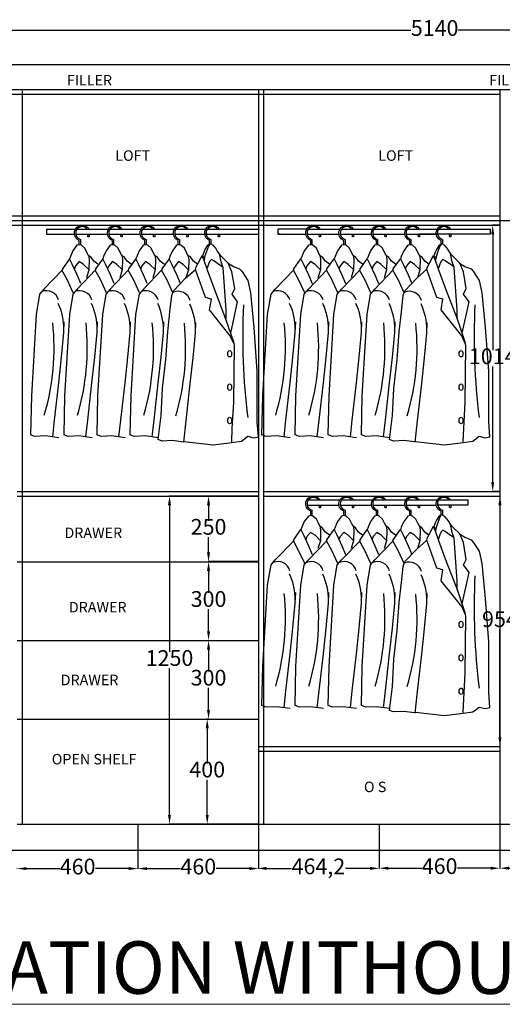
# Model space of a CAD drawing. Units: millimetres. Extents: x 1304 to 14372, y 283 to 7516.
# Tile 2 of 4: x 3237 to 5077, y 283 to 4036. Entities that reach past the tile are written whole.
import ezdxf

# ---------------------------------------------------------------- set-up
doc = ezdxf.new("R2010")
doc.units = ezdxf.units.MM
doc.layers.get('Defpoints').update_dxf_attribs({"color": 2})
for name, color, linetype, lineweight in [('A-ANNO-DIMS', 2, 'Continuous', 18), ('A-ANNO-TEXT', 3, 'Continuous', 18), ('A-FURN', 7, 'Continuous', 25)]:
    doc.layers.add(name, color=color, linetype=linetype, lineweight=lineweight)
doc.styles.get("Standard").update_dxf_attribs({"font": 'arial.ttf'})
doc.dimstyles.new('ISO-25', dxfattribs={"dimtxt": 60, "dimasz": 35, "dimexe": 1.25, "dimexo": 0.625, "dimtad": 0, "dimtih": 1, "dimtoh": 1, "dimtxsty": 'Standard', "dimcen": 2.5, "dimclrd": 1, "dimclre": 3, "dimadec": 0, "dimazin": 0, "dimtfac": 1, "dimtmove": 0, "dimatfit": 3, "dimfxl": 1, "dimarcsym": 0})

# ---------------------------------------------------------------- blocks, each defined once
blk = doc.blocks.new('*D16')
at = {"layer": 'A-ANNO-DIMS', "color": 0, "lineweight": -2, "transparency": 16777216}
for p, q in [((2248.6, 4008), (2248.6, 3995.4)), ((2283.6, 3996.6), (4728.5, 3996.6)), ((7353.6, 3996.6), (4908.8, 3996.6)), ((7388.6, 3865.9), (7388.6, 3997.9))]:
    blk.add_line(p, q, dxfattribs=at)
at = {"layer": 'A-ANNO-DIMS', "color": 0, "transparency": 16777216}
for points in [[(2283.6, 4002.4), (2283.6, 3990.8), (2248.6, 3996.6)], [(7353.6, 4002.4), (7353.6, 3990.8), (7388.6, 3996.6)]]:
    blk.add_solid(points, dxfattribs=at)
at = {"layer": 'Defpoints', "color": 0, "transparency": 16777216}
for p in [(2248.6, 4008.6), (7388.6, 3996.6), (7388.6, 3865.3)]:
    blk.add_point(p, dxfattribs=at)
at = {"layer": 'A-ANNO-DIMS', "color": 0, "transparency": 16777216, "insert": (4818.6, 3996.6), "char_height": 60, "attachment_point": 5}
blk.add_mtext('5140', dxfattribs=at)
blk = doc.blocks.new('*D18')
at = {"layer": 'A-ANNO-DIMS', "color": 0, "lineweight": -2, "transparency": 16777216}
for p, q in [((4147, 2220.3), (3955.4, 2220.3)), ((3956.7, 2185.3), (3956.7, 2126.5)), ((3956.7, 2005.3), (3956.7, 2064)), ((4147, 1970.3), (3955.4, 1970.3))]:
    blk.add_line(p, q, dxfattribs=at)
at = {"layer": 'A-ANNO-DIMS', "color": 0, "transparency": 16777216}
for points in [[(3950.8, 2185.3), (3962.5, 2185.3), (3956.7, 2220.3)], [(3950.8, 2005.3), (3962.5, 2005.3), (3956.7, 1970.3)]]:
    blk.add_solid(points, dxfattribs=at)
at = {"layer": 'Defpoints', "color": 0, "transparency": 16777216}
for p in [(4147.6, 2220.3), (3956.7, 1970.3), (4147.6, 1970.3)]:
    blk.add_point(p, dxfattribs=at)
at = {"layer": 'A-ANNO-DIMS', "color": 0, "transparency": 16777216, "insert": (3956.7, 2095.3), "char_height": 60, "attachment_point": 5}
blk.add_mtext('250', dxfattribs=at)
blk = doc.blocks.new('*D19')
at = {"layer": 'A-ANNO-DIMS', "color": 0, "lineweight": -2, "transparency": 16777216}
for p, q in [((3957.3, 1970.3), (3957.9, 1970.3)), ((3956.7, 1935.3), (3956.7, 1851.6)), ((3956.7, 1705.3), (3956.7, 1789)), ((3957.3, 1670.3), (3957.9, 1670.3))]:
    blk.add_line(p, q, dxfattribs=at)
at = {"layer": 'A-ANNO-DIMS', "color": 0, "transparency": 16777216}
for points in [[(3950.8, 1935.3), (3962.5, 1935.3), (3956.7, 1970.3)], [(3950.8, 1705.3), (3962.5, 1705.3), (3956.7, 1670.3)]]:
    blk.add_solid(points, dxfattribs=at)
at = {"layer": 'Defpoints', "color": 0, "transparency": 16777216}
for p in [(3956.7, 1970.3), (3956.7, 1670.3), (3956.7, 1670.3)]:
    blk.add_point(p, dxfattribs=at)
at = {"layer": 'A-ANNO-DIMS', "color": 0, "transparency": 16777216, "insert": (3956.7, 1820.3), "char_height": 60, "attachment_point": 5}
blk.add_mtext('300', dxfattribs=at)
blk = doc.blocks.new('*D20')
at = {"layer": 'A-ANNO-DIMS', "color": 0, "lineweight": -2, "transparency": 16777216}
for p, q in [((3957.3, 1670.3), (3957.9, 1670.3)), ((3956.7, 1635.3), (3956.7, 1551.6)), ((3956.7, 1405.3), (3956.7, 1489)), ((3957.3, 1370.3), (3957.9, 1370.3))]:
    blk.add_line(p, q, dxfattribs=at)
at = {"layer": 'A-ANNO-DIMS', "color": 0, "transparency": 16777216}
for points in [[(3950.8, 1635.3), (3962.5, 1635.3), (3956.7, 1670.3)], [(3950.8, 1405.3), (3962.5, 1405.3), (3956.7, 1370.3)]]:
    blk.add_solid(points, dxfattribs=at)
at = {"layer": 'Defpoints', "color": 0, "transparency": 16777216}
for p in [(3956.7, 1670.3), (3956.7, 1370.3), (3956.7, 1370.3)]:
    blk.add_point(p, dxfattribs=at)
at = {"layer": 'A-ANNO-DIMS', "color": 0, "transparency": 16777216, "insert": (3956.7, 1520.3), "char_height": 60, "attachment_point": 5}
blk.add_mtext('300', dxfattribs=at)
blk = doc.blocks.new('*D21')
at = {"layer": 'A-ANNO-DIMS', "color": 0, "lineweight": -2, "transparency": 16777216}
for p, q in [((3957.3, 1370.3), (3950.3, 1370.3)), ((3951.6, 1335.3), (3951.6, 1201.5)), ((3951.6, 1005.3), (3951.6, 1139)), ((3957.3, 970.3), (3950.3, 970.3))]:
    blk.add_line(p, q, dxfattribs=at)
at = {"layer": 'A-ANNO-DIMS', "color": 0, "transparency": 16777216}
for points in [[(3945.7, 1335.3), (3957.4, 1335.3), (3951.6, 1370.3)], [(3945.7, 1005.3), (3957.4, 1005.3), (3951.6, 970.3)]]:
    blk.add_solid(points, dxfattribs=at)
at = {"layer": 'Defpoints', "color": 0, "transparency": 16777216}
for p in [(3957.9, 1370.3), (3951.6, 970.3), (3957.9, 970.3)]:
    blk.add_point(p, dxfattribs=at)
at = {"layer": 'A-ANNO-DIMS', "color": 0, "transparency": 16777216, "insert": (3951.6, 1170.3), "char_height": 60, "attachment_point": 5}
blk.add_mtext('400', dxfattribs=at)
blk = doc.blocks.new('*D22')
at = {"layer": 'A-ANNO-DIMS', "color": 0, "lineweight": -2, "transparency": 16777216}
for p, q in [((4147, 2220.3), (3806.5, 2220.3)), ((3807.8, 2185.3), (3807.8, 1626.5)), ((3807.8, 1005.3), (3807.8, 1564)), ((4147, 970.3), (3806.5, 970.3))]:
    blk.add_line(p, q, dxfattribs=at)
at = {"layer": 'A-ANNO-DIMS', "color": 0, "transparency": 16777216}
for points in [[(3801.9, 2185.3), (3813.6, 2185.3), (3807.8, 2220.3)], [(3801.9, 1005.3), (3813.6, 1005.3), (3807.8, 970.3)]]:
    blk.add_solid(points, dxfattribs=at)
at = {"layer": 'Defpoints', "color": 0, "transparency": 16777216}
for p in [(4147.6, 2220.3), (3807.8, 970.3), (4147.6, 970.3)]:
    blk.add_point(p, dxfattribs=at)
at = {"layer": 'A-ANNO-DIMS', "color": 0, "transparency": 16777216, "insert": (3807.8, 1595.3), "char_height": 60, "attachment_point": 5}
blk.add_mtext('1250', dxfattribs=at)
blk = doc.blocks.new('*D23')
at = {"layer": 'A-ANNO-DIMS', "color": 0, "lineweight": -2, "transparency": 16777216}
for p, q in [((5067, 3252.3), (5038.8, 3252.3)), ((5040.1, 3217.3), (5040.1, 2776.5)), ((5040.1, 2273.3), (5040.1, 2714)), ((5067, 2238.3), (5038.8, 2238.3))]:
    blk.add_line(p, q, dxfattribs=at)
at = {"layer": 'A-ANNO-DIMS', "color": 0, "transparency": 16777216}
for points in [[(5034.2, 3217.3), (5045.9, 3217.3), (5040.1, 3252.3)], [(5034.2, 2273.3), (5045.9, 2273.3), (5040.1, 2238.3)]]:
    blk.add_solid(points, dxfattribs=at)
at = {"layer": 'Defpoints', "color": 0, "transparency": 16777216}
for p in [(5067.6, 3252.3), (5040.1, 2238.3), (5067.6, 2238.3)]:
    blk.add_point(p, dxfattribs=at)
at = {"layer": 'A-ANNO-DIMS', "color": 0, "transparency": 16777216, "insert": (5040.1, 2745.3), "char_height": 60, "attachment_point": 5}
blk.add_mtext('1014', dxfattribs=at)
blk = doc.blocks.new('*D24')
at = {"layer": 'A-ANNO-DIMS', "color": 0, "lineweight": -2, "transparency": 16777216}
for p, q in [((5068.3, 2220.3), (5068.9, 2220.3)), ((5067.6, 2185.3), (5067.6, 1774.5)), ((5067.6, 1301.3), (5067.6, 1712)), ((5068.3, 1266.3), (5068.9, 1266.3))]:
    blk.add_line(p, q, dxfattribs=at)
at = {"layer": 'A-ANNO-DIMS', "color": 0, "transparency": 16777216}
for points in [[(5061.8, 2185.3), (5073.5, 2185.3), (5067.6, 2220.3)], [(5061.8, 1301.3), (5073.5, 1301.3), (5067.6, 1266.3)]]:
    blk.add_solid(points, dxfattribs=at)
at = {"layer": 'Defpoints', "color": 0, "transparency": 16777216}
for p in [(5067.6, 2220.3), (5067.6, 1266.3), (5067.6, 1266.3)]:
    blk.add_point(p, dxfattribs=at)
at = {"layer": 'A-ANNO-DIMS', "color": 0, "transparency": 16777216, "insert": (5067.6, 1743.3), "char_height": 60, "attachment_point": 5}
blk.add_mtext('954', dxfattribs=at)
blk = doc.blocks.new('*D36')
at = {"layer": 'A-ANNO-DIMS', "color": 0, "lineweight": -2, "transparency": 16777216}
for p, q in [((3227.6, 801.1), (3227.6, 801.7)), ((3262.6, 800.5), (3389.6, 800.5)), ((3652.6, 800.5), (3525.7, 800.5)), ((3687.6, 801.1), (3687.6, 801.7))]:
    blk.add_line(p, q, dxfattribs=at)
at = {"layer": 'A-ANNO-DIMS', "color": 0, "transparency": 16777216}
for points in [[(3262.6, 806.3), (3262.6, 794.7), (3227.6, 800.5)], [(3652.6, 806.3), (3652.6, 794.7), (3687.6, 800.5)]]:
    blk.add_solid(points, dxfattribs=at)
at = {"layer": 'Defpoints', "color": 0, "transparency": 16777216}
for p in [(3227.6, 800.5), (3687.6, 800.5), (3687.6, 800.5)]:
    blk.add_point(p, dxfattribs=at)
at = {"layer": 'A-ANNO-DIMS', "color": 0, "transparency": 16777216, "insert": (3457.6, 800.5), "char_height": 60, "attachment_point": 5}
blk.add_mtext('460', dxfattribs=at)
blk = doc.blocks.new('*D37')
at = {"layer": 'A-ANNO-DIMS', "color": 0, "lineweight": -2, "transparency": 16777216}
for p, q in [((4143.4, 801.8), (4143.4, 802.4)), ((4178.4, 801.2), (4272.8, 801.2)), ((4572.6, 801.2), (4478.3, 801.2)), ((4607.6, 801.8), (4607.6, 802.4))]:
    blk.add_line(p, q, dxfattribs=at)
at = {"layer": 'A-ANNO-DIMS', "color": 0, "transparency": 16777216}
for points in [[(4178.4, 807), (4178.4, 795.4), (4143.4, 801.2)], [(4572.6, 807), (4572.6, 795.4), (4607.6, 801.2)]]:
    blk.add_solid(points, dxfattribs=at)
at = {"layer": 'Defpoints', "color": 0, "transparency": 16777216}
for p in [(4143.4, 801.2), (4607.6, 801.2), (4607.6, 801.2)]:
    blk.add_point(p, dxfattribs=at)
at = {"layer": 'A-ANNO-DIMS', "color": 0, "transparency": 16777216, "insert": (4375.5, 801.2), "char_height": 60, "attachment_point": 5}
blk.add_mtext('464,2', dxfattribs=at)
blk = doc.blocks.new('*D38')
at = {"layer": 'A-ANNO-DIMS', "color": 0, "lineweight": -2, "transparency": 16777216}
for p, q in [((4607.6, 969.7), (4607.6, 800.7)), ((5067.6, 969.7), (5067.6, 800.7)), ((4642.6, 802), (4769.6, 802)), ((5032.6, 802), (4905.7, 802))]:
    blk.add_line(p, q, dxfattribs=at)
at = {"layer": 'A-ANNO-DIMS', "color": 0, "transparency": 16777216}
for points in [[(4642.6, 807.8), (4642.6, 796.1), (4607.6, 802)], [(5032.6, 807.8), (5032.6, 796.1), (5067.6, 802)]]:
    blk.add_solid(points, dxfattribs=at)
at = {"layer": 'Defpoints', "color": 0, "transparency": 16777216}
for p in [(4607.6, 970.3), (5067.6, 970.3), (5067.6, 802)]:
    blk.add_point(p, dxfattribs=at)
at = {"layer": 'A-ANNO-DIMS', "color": 0, "transparency": 16777216, "insert": (4837.6, 802), "char_height": 60, "attachment_point": 5}
blk.add_mtext('460', dxfattribs=at)
blk = doc.blocks.new('*D39')
at = {"layer": 'A-ANNO-DIMS', "color": 0, "lineweight": -2, "transparency": 16777216}
for p, q in [((5067.6, 969.7), (5067.6, 800.7)), ((5527.6, 969.7), (5527.6, 800.7)), ((5102.6, 802), (5229.6, 802)), ((5492.6, 802), (5365.7, 802))]:
    blk.add_line(p, q, dxfattribs=at)
at = {"layer": 'A-ANNO-DIMS', "color": 0, "transparency": 16777216}
for points in [[(5102.6, 807.8), (5102.6, 796.1), (5067.6, 802)], [(5492.6, 807.8), (5492.6, 796.1), (5527.6, 802)]]:
    blk.add_solid(points, dxfattribs=at)
at = {"layer": 'Defpoints', "color": 0, "transparency": 16777216}
for p in [(5067.6, 970.3), (5527.6, 970.3), (5527.6, 802)]:
    blk.add_point(p, dxfattribs=at)
at = {"layer": 'A-ANNO-DIMS', "color": 0, "transparency": 16777216, "insert": (5297.6, 802), "char_height": 60, "attachment_point": 5}
blk.add_mtext('460', dxfattribs=at)
blk = doc.blocks.new('*D44')
at = {"layer": 'A-ANNO-DIMS', "color": 0, "lineweight": -2, "transparency": 16777216}
for p, q in [((3687.6, 969.7), (3687.6, 799.2)), ((4147.6, 969.7), (4147.6, 799.2)), ((3722.6, 800.5), (3849.6, 800.5)), ((4112.6, 800.5), (3985.7, 800.5))]:
    blk.add_line(p, q, dxfattribs=at)
at = {"layer": 'A-ANNO-DIMS', "color": 0, "transparency": 16777216}
for points in [[(3722.6, 806.3), (3722.6, 794.7), (3687.6, 800.5)], [(4112.6, 806.3), (4112.6, 794.7), (4147.6, 800.5)]]:
    blk.add_solid(points, dxfattribs=at)
at = {"layer": 'Defpoints', "color": 0, "transparency": 16777216}
for p in [(3687.6, 970.3), (4147.6, 970.3), (3687.6, 800.5)]:
    blk.add_point(p, dxfattribs=at)
at = {"layer": 'A-ANNO-DIMS', "color": 0, "transparency": 16777216, "insert": (3917.6, 800.5), "char_height": 60, "attachment_point": 5}
blk.add_mtext('460', dxfattribs=at)
blk = doc.blocks.new('CLOTHES-HANGING')
for p, q in [((4337.7, 3238.2), (4457.6, 3238.2)), ((4463.8, 3238.2), (4582, 3238.2)), ((4588.1, 3238.2), (4709.1, 3238.2)), ((4715.2, 3238.2), (4828.6, 3238.2)), ((4332.7, 3218.2), (4453.7, 3218.2)), ((4458.7, 3218.2), (4578, 3218.2)), ((4583.1, 3218.2), (4705.1, 3218.2)), ((4710.2, 3218.2), (4824.6, 3218.2))]:
    blk.add_line(p, q)
for points in [[(4346, 3177.2), (4346, 3194.9, -0.375799), (4328.2, 3230.2, -0.662316), (4381.8, 3238.2), (4421.2, 3238.2)], [(4375.7, 3238.2, 0.616313), (4333.1, 3229, 0.413702), (4351, 3198.5), (4351, 3177.2)], [(4472, 3177.2), (4472, 3194.9, -0.375799), (4454.3, 3230.2, -0.662316), (4507.9, 3238.2)], [(4501.8, 3238.2, 0.616313), (4459.1, 3229, 0.413702), (4477, 3198.5), (4477, 3177.2)], [(4596.4, 3177.2), (4596.4, 3194.9, -0.375799), (4578.7, 3230.2, -0.662316), (4632.3, 3238.2)], [(4626.1, 3238.2, 0.616313), (4583.5, 3229, 0.413702), (4601.4, 3198.5), (4601.4, 3177.2)], [(4723.5, 3177.6), (4723.5, 3194.9, -0.375799), (4705.7, 3230.2, -0.662316), (4759.3, 3238.2)], [(4753.2, 3238.2, 0.616313), (4710.6, 3229, 0.413702), (4728.5, 3198.5), (4728.5, 3178)], [(4843, 3179.9), (4843, 3194.9, -0.375799), (4825.2, 3230.2, -0.662316), (4878.8, 3238.2)], [(4872.7, 3238.2, 0.616313), (4830.1, 3229, 0.413702), (4848, 3198.5), (4848, 3180.3)], [(4383.5, 3218.2, -0.068798), (4383.9, 3210.2, -1.055238), (4378.9, 3210.6, 0.07858), (4378.4, 3218.2, 0.07858)], [(4509.5, 3218.2, -0.068798), (4509.9, 3210.2, -1.055238), (4504.9, 3210.6, 0.07858), (4504.4, 3218.2)], [(4633.9, 3218.2, -0.068798), (4634.3, 3210.2, -1.055238), (4629.3, 3210.6, 0.07858), (4628.8, 3218.2)], [(4761, 3218.2, -0.068798), (4761.4, 3210.2, -1.055238), (4756.4, 3210.6, 0.07858), (4755.9, 3218.2)], [(4880.4, 3218.2, -0.068798), (4880.8, 3210.2, -1.055238), (4875.8, 3210.6, 0.07858), (4875.3, 3218.2)]]:
    blk.add_lwpolyline(points, format="xyb")
for points in [[(4381.1, 3137), (4375.4, 3148.9), (4367.7, 3164.8), (4354.3, 3176.3), (4346.7, 3178.2), (4337.1, 3176.3), (4321.8, 3155.3), (4312.3, 3133.6), (4309.1, 3124)], [(4507.8, 3137), (4502, 3148.9), (4494.4, 3164.8), (4481, 3176.3), (4473.3, 3178.2), (4463.8, 3176.3), (4448.5, 3155.3), (4438.9, 3133.6), (4435.7, 3124)], [(4633.8, 3137), (4628.1, 3148.9), (4620.4, 3164.8), (4607, 3176.3), (4599.4, 3178.2), (4589.8, 3176.3), (4574.5, 3155.3), (4565, 3133.6), (4561.8, 3124)], [(4760.5, 3137), (4754.7, 3148.9), (4747.1, 3164.8), (4733.7, 3176.3), (4726, 3178.2), (4716.5, 3176.3), (4701.2, 3155.3), (4691.6, 3133.6), (4688.4, 3124)], [(4844.1, 3180.6), (4834, 3174), (4825.2, 3160.3), (4820.3, 3149.8), (4815.3, 3134.5)], [(4905.1, 2895.5), (4905.1, 2928.3), (4893.2, 3092), (4885.8, 3113.6), (4879.5, 3145.3), (4872.3, 3155.4), (4866.4, 3164.6), (4857.9, 3174.7), (4848.7, 3179.9), (4844.1, 3180.6), (4838.9, 3172.4), (4830.7, 3152.1), (4825.2, 3135.8), (4821.9, 3121.7), (4821.6, 3119.8)], [(4268.3, 2442.4), (4216.9, 2449.4), (4176.8, 2447.6), (4160, 2453.9), (4163.3, 2602.1), (4181.5, 2912.1), (4194.8, 2990.1), (4211.2, 3009.3), (4281.6, 3082.3), (4281.6, 3085.9), (4309, 3124.3), (4319, 3104.2), (4338.2, 3063.1), (4352.3, 3030.2)], [(4395, 2442.4), (4343.5, 2449.4), (4303.4, 2447.6), (4286.6, 2453.9), (4289.9, 2602.1), (4308.2, 2912.1), (4321.5, 2990.1), (4337.9, 3009.3), (4408.2, 3082.3), (4408.2, 3085.9), (4435.6, 3124.3), (4445.7, 3104.2), (4464.8, 3063.1), (4479, 3030.2)], [(4417.3, 3103.8), (4402.1, 3115.1), (4390.2, 3131.6), (4381.1, 3137), (4383.9, 3123.3), (4382.9, 3082.3), (4373.4, 3051.9)], [(4521, 2442.4), (4469.6, 2449.4), (4429.5, 2447.6), (4412.7, 2453.9), (4416, 2602.1), (4434.2, 2912.1), (4447.5, 2990.1), (4463.9, 3009.3), (4534.3, 3082.3), (4534.3, 3085.9), (4561.7, 3124.3), (4571.7, 3104.2), (4590.9, 3063.1), (4605, 3030.2)], [(4543.9, 3103.8), (4528.8, 3115.1), (4516.9, 3131.6), (4507.8, 3137), (4510.5, 3123.3), (4509.6, 3082.3), (4500.1, 3051.9)], [(4647.7, 2442.4), (4596.2, 2449.4), (4556.1, 2447.6), (4539.3, 2453.9), (4542.6, 2602.1), (4560.9, 2912.1), (4574.2, 2990.1), (4590.6, 3009.3), (4660.9, 3082.3), (4660.9, 3085.9), (4688.3, 3124.3), (4698.4, 3104.2), (4717.5, 3063.1), (4731.7, 3030.2)], [(4670, 3103.8), (4654.8, 3115.1), (4642.9, 3131.6), (4633.8, 3137), (4636.6, 3123.3), (4635.6, 3082.3), (4626.1, 3051.9)], [(4741.7, 2426.4), (4701.6, 2431.8), (4661.5, 2430), (4646.8, 2435.5), (4657.7, 2527.1), (4662.8, 2630.8), (4676.4, 2741.2), (4683.2, 2846.6), (4691.7, 2923.1), (4698.5, 2984.2), (4705.3, 3002.9), (4751.3, 3050.5), (4788.7, 3084.5), (4791.6, 3094), (4800.3, 3110.8), (4810.1, 3129.9), (4814.2, 3136.2), (4822.9, 3129.9), (4824, 3129.3)], [(4796.6, 3103.8), (4781.5, 3115.1), (4769.6, 3131.6), (4760.5, 3137), (4763.2, 3123.3), (4762.3, 3082.3), (4752.8, 3051.9)], [(4813, 3134.5), (4820.5, 3120), (4833.9, 3083), (4858.8, 3013.5), (4903.9, 2896.1), (4934, 2808.5), (4936.1, 2793.8), (4933.4, 2577.1), (4928.1, 2479.6), (4926.4, 2426.9)], [(4891.3, 3093.9), (4878.5, 3102.4), (4858.9, 3116.8), (4850.4, 3122.1), (4843.8, 3115.8), (4838.3, 3104.7), (4834.7, 3092.6), (4833.3, 3088.4)], [(4923.7, 2841.2), (4949.8, 2961), (4929, 2990.1), (4939.4, 3010.9), (4928.2, 3074.9), (4914.1, 3108.4), (4888.7, 3132.9), (4877.6, 3145.6)], [(4323.2, 2995.2), (4300.2, 3045.3), (4280.1, 3081.8)], [(4383.7, 3082), (4362.6, 3103), (4345.4, 3113.9), (4332, 3097.9), (4327.4, 3086.3)], [(4449.8, 2995.2), (4426.8, 3045.3), (4406.8, 3081.8)], [(4510.3, 3082), (4489.3, 3103), (4472.1, 3113.9), (4458.7, 3097.9), (4454, 3086.3)], [(4575.9, 2995.2), (4552.9, 3045.3), (4532.8, 3081.8)], [(4636.4, 3082), (4615.3, 3103), (4598.1, 3113.9), (4584.7, 3097.9), (4580.1, 3086.3)], [(4702.5, 2995.2), (4679.5, 3045.3), (4659.4, 3081.8)], [(4763, 3082), (4742, 3103), (4724.8, 3113.9), (4711.4, 3097.9), (4706.7, 3086.3)], [(4935, 2802.3), (4921.9, 2831), (4842.9, 2929.7), (4849.5, 2970.8), (4827.3, 2977.3), (4789.4, 3084.2)], [(4913.3, 3108.4), (4934.2, 3095.7), (4957.3, 3086), (4965.4, 3077.1), (4988.3, 3042.5), (4998.2, 2994.9), (5011, 2862.2), (5023.4, 2696.6), (5023.4, 2503.8), (5027.9, 2446.2)], [(4244.7, 2445.6), (4251.6, 2509.4), (4267.7, 2651.6), (4278.3, 2749.4), (4287.2, 2843.6), (4289, 2884.5)], [(4371.4, 2445.6), (4378.3, 2509.4), (4394.3, 2651.6), (4405, 2749.4), (4413.9, 2843.6), (4415.7, 2884.5)], [(4497.4, 2445.6), (4504.3, 2509.4), (4520.4, 2651.6), (4531, 2749.4), (4539.9, 2843.6), (4541.7, 2884.5)], [(4624, 2445.6), (4631, 2509.4), (4647, 2651.6), (4657.7, 2749.4), (4666.6, 2843.6), (4668.4, 2884.5)], [(4744.4, 2425.4), (4753.3, 2507.2), (4769.3, 2649.4), (4779.9, 2747.1), (4788.8, 2841.3), (4790.6, 2882.2)], [(4745.3, 2428.2), (4856.5, 2415.4), (4927.6, 2424.5), (4964.1, 2430), (4988.3, 2448.2), (5011.3, 2442.8), (5029, 2446.4)]]:
    blk.add_lwpolyline(points)
for centre, radius, start, end in [((4220.5, 2954.5), 48.4, 15.7523, 111.1565), ((4347.2, 2954.5), 48.4, 15.7523, 111.1565), ((4473.2, 2954.5), 48.4, 15.7523, 111.1565), ((4599.9, 2954.5), 48.4, 15.7523, 111.1565), ((4722.1, 2952.3), 48.4, 15.7523, 111.1565), ((4054.1, 2856), 233.4, 359.9116, 24.988), ((4180.8, 2856), 233.4, 359.9116, 24.988), ((4306.8, 2856), 233.4, 359.9116, 24.988), ((4433.5, 2856), 233.4, 359.9116, 24.988), ((4555.7, 2853.8), 233.4, 359.9116, 24.988), ((7480.3, 2829.3), 2511.1, 177.2767, 187.0811), ((3340.3, 2786.1), 909.7, 343.5409, 5.9886), ((3466.9, 2786.1), 909.7, 343.5409, 5.9886), ((3719.6, 2786.1), 909.7, 343.5409, 5.9886), ((3841.9, 2783.9), 909.7, 343.5409, 5.9886)]:
    blk.add_arc(centre, radius, start, end)
for centre in [(4919.4, 2762.9), (4919.4, 2635.5), (4919.4, 2508.1)]:
    blk.add_ellipse(centre, major_axis=(0, 12.4), ratio=0.580645)

msp = doc.modelspace()

# ---------------------------------------------------------------- linework, layer by layer
at = {"layer": 'A-FURN'}
for p, q in [((2018.643, 3865.285), (7618.643, 3865.285)), ((2316.643, 3770.285), (7388.643, 3770.285)), ((3245.643, 3765.285), (3245.643, 970.285)), ((4147.643, 3770.285), (4147.643, 970.285)), ((4165.643, 3770.285), (4165.643, 970.285)), ((5067.643, 3770.285), (5067.643, 970.285)), ((2316.643, 3752.285), (5067.643, 3752.285)), ((2316.643, 3288.285), (5067.643, 3288.285)), ((2316.643, 3270.285), (5545.643, 3270.285)), ((2316.643, 3252.285), (4165.643, 3252.285)), ((3339.108, 3238.199), (3449.429, 3238.199)), ((3339.108, 3238.199), (3339.108, 3218.199)), ((3455.532, 3238.199), (3575.461, 3238.199)), ((3499.644, 3238.199), (3538.99, 3238.199)), ((3581.563, 3238.199), (3699.848, 3238.199)), ((3705.951, 3238.199), (3826.926, 3238.199)), ((3833.029, 3238.199), (3946.395, 3238.199)), ((3881.136, 3238.199), (4147.643, 3238.199)), ((4165.643, 3252.285), (5067.643, 3252.285)), ((3339.108, 3218.199), (3445.437, 3218.199)), ((3450.506, 3218.199), (3571.468, 3218.199)), ((3576.537, 3218.199), (3695.856, 3218.199)), ((3700.925, 3218.199), (3822.934, 3218.199)), ((3828.003, 3218.199), (3942.403, 3218.199)), ((3876.11, 3218.199), (4147.643, 3218.199)), ((4229.579, 3218.199), (4221.295, 3218.199)), ((3227.643, 2238.285), (4147.643, 2238.285)), ((3227.643, 2220.285), (4147.643, 2220.285)), ((4165.643, 2238.285), (5067.643, 2238.285)), ((4165.643, 2220.285), (5067.643, 2220.285)), ((4945.153, 2186.199), (4829.663, 2186.177)), ((4834.685, 2206.199), (4945.153, 2206.199)), ((4945.153, 2206.199), (4945.153, 2186.199)), ((3227.643, 1970.285), (4147.643, 1970.285)), ((3227.643, 1670.285), (4147.643, 1670.285)), ((3227.643, 1370.285), (4147.643, 1370.285)), ((4147.643, 1266.285), (5067.643, 1266.285)), ((4147.643, 1248.285), (5067.643, 1248.285)), ((3227.643, 970.285), (4147.643, 970.285)), ((4147.643, 970.285), (5527.643, 970.285)), ((2018.643, 870.285), (7618.643, 870.285))]:
    msp.add_line(p, q, dxfattribs=at)
for points in [[(3463.826, 3177.2), (3463.826, 3194.87, -0.37579854), (3446.056, 3230.24, -0.66231577), (3499.644, 3238.199, -0.66231577)], [(3493.542, 3238.199, 0.61631348), (3450.897, 3228.987, 0.41370242), (3468.826, 3198.466), (3468.826, 3177.234)], [(3589.858, 3177.2), (3589.858, 3194.87, -0.37579854), (3572.088, 3230.24, -0.66231577), (3625.676, 3238.199)], [(3619.573, 3238.199, 0.61631348), (3576.928, 3228.987, 0.41370242), (3594.858, 3198.466), (3594.858, 3177.234)], [(3714.245, 3177.2), (3714.245, 3194.87, -0.37579854), (3696.475, 3230.24, -0.66231577), (3750.063, 3238.199)], [(3743.961, 3238.199, 0.61631348), (3701.316, 3228.987, 0.41370242), (3719.245, 3198.466), (3719.245, 3177.234)], [(3841.323, 3177.573), (3841.323, 3194.87, -0.37579854), (3823.554, 3230.24, -0.66231577), (3877.141, 3238.199)], [(3871.039, 3238.199, 0.61631348), (3828.394, 3228.987, 0.41370242), (3846.323, 3198.466), (3846.323, 3177.951)], [(3960.792, 3179.875), (3960.792, 3194.87, -0.37579854), (3943.022, 3230.24, -0.66231577), (3996.61, 3238.199)], [(3990.508, 3238.199, 0.61631348), (3947.863, 3228.987, 0.41370242), (3965.792, 3198.466), (3965.792, 3180.349)], [(3501.277, 3218.199, -0.06879847), (3501.677, 3210.151, -1.05523784), (3496.696, 3210.589, 0.07858039), (3496.169, 3218.199, 0.07858039)], [(3627.308, 3218.199, -0.06879847), (3627.709, 3210.151, -1.05523784), (3622.728, 3210.589, 0.07858039), (3622.201, 3218.199)], [(3751.696, 3218.199, -0.06879847), (3752.096, 3210.151, -1.05523784), (3747.115, 3210.589, 0.07858039), (3746.588, 3218.199)], [(3878.774, 3218.199, -0.06879847), (3879.174, 3210.151, -1.05523784), (3874.193, 3210.589, 0.07858039), (3873.666, 3218.199)], [(3998.242, 3218.199, -0.06879847), (3998.643, 3210.151, -1.05523784), (3993.662, 3210.589, 0.07858039), (3993.135, 3218.199)]]:
    msp.add_lwpolyline(points, format="xyb", dxfattribs=at)
for points in [[(4331.617, 3238.199), (4221.295, 3238.199), (4221.295, 3218.199), (4327.624, 3218.199)], [(4763.323, 3238.199), (5029.83, 3238.199), (5029.83, 3218.199), (4758.297, 3218.199)], [(3498.925, 3137.031), (3493.189, 3148.886), (3485.539, 3164.81), (3472.151, 3176.276), (3464.501, 3178.186), (3454.939, 3176.276), (3439.639, 3155.256), (3430.076, 3133.599), (3426.889, 3124.045)], [(3625.574, 3137.031), (3619.837, 3148.886), (3612.187, 3164.81), (3598.8, 3176.276), (3591.15, 3178.186), (3581.587, 3176.276), (3566.287, 3155.256), (3556.725, 3133.599), (3553.537, 3124.045)], [(3751.624, 3137.031), (3745.887, 3148.886), (3738.237, 3164.81), (3724.85, 3176.276), (3717.2, 3178.186), (3707.637, 3176.276), (3692.337, 3155.256), (3682.775, 3133.599), (3679.587, 3124.045)], [(3878.272, 3137.031), (3872.536, 3148.886), (3864.886, 3164.81), (3851.498, 3176.276), (3843.848, 3178.186), (3834.286, 3176.276), (3818.986, 3155.256), (3809.423, 3133.599), (3806.236, 3124.045)], [(3961.959, 3180.587), (3951.813, 3174.046), (3942.976, 3160.312), (3938.066, 3149.847), (3933.157, 3134.477)], [(3997.307, 3145.269), (3990.107, 3155.406), (3984.215, 3164.563), (3975.705, 3174.7), (3966.541, 3179.933), (3961.959, 3180.587), (3956.722, 3172.411), (3948.54, 3152.136), (3942.976, 3135.785), (3939.703, 3121.723), (3939.375, 3119.761)], [(3470.126, 3030.195), (3456.003, 3063.121), (3436.825, 3104.182), (3426.779, 3124.256), (3399.381, 3085.933), (3399.381, 3082.283), (3329.062, 3009.285), (3312.623, 2990.123), (3299.345, 2912.137), (3281.091, 2602.085), (3277.795, 2453.884)], [(3596.774, 3030.195), (3582.651, 3063.121), (3563.473, 3104.182), (3553.427, 3124.256), (3526.03, 3085.933), (3526.03, 3082.283), (3455.71, 3009.285), (3439.272, 2990.123), (3425.993, 2912.137), (3407.739, 2602.085), (3404.443, 2453.884)], [(3535.105, 3103.76), (3519.93, 3115.132), (3508.058, 3131.556), (3498.925, 3137.031), (3501.665, 3123.344), (3500.752, 3082.283), (3491.243, 3051.881)], [(3722.824, 3030.195), (3708.701, 3063.121), (3689.523, 3104.182), (3679.477, 3124.256), (3652.08, 3085.933), (3652.08, 3082.283), (3581.76, 3009.285), (3565.322, 2990.123), (3552.043, 2912.137), (3533.789, 2602.085), (3530.493, 2453.884)], [(3661.753, 3103.76), (3646.578, 3115.132), (3634.706, 3131.556), (3625.574, 3137.031), (3628.313, 3123.344), (3627.4, 3082.283), (3617.892, 3051.881)], [(3849.473, 3030.195), (3835.35, 3063.121), (3816.171, 3104.182), (3806.126, 3124.256), (3778.728, 3085.933), (3778.728, 3082.283), (3708.409, 3009.285), (3691.97, 2990.123), (3678.692, 2912.137), (3660.438, 2602.085), (3657.142, 2453.884)], [(3787.803, 3103.76), (3772.628, 3115.132), (3760.756, 3131.556), (3751.624, 3137.031), (3754.363, 3123.344), (3753.45, 3082.283), (3743.942, 3051.881)], [(3764.654, 2435.499), (3775.536, 2527.141), (3780.638, 2630.794), (3794.244, 2741.244), (3801.046, 2846.596), (3809.55, 2923.061), (3816.352, 2984.234), (3823.155, 3002.925), (3869.073, 3050.504), (3906.488, 3084.488), (3909.388, 3093.978), (3918.076, 3110.76), (3927.922, 3129.857), (3931.976, 3136.223), (3940.664, 3129.857), (3941.822, 3129.278)], [(3914.452, 3103.76), (3899.277, 3115.132), (3887.404, 3131.556), (3878.272, 3137.031), (3881.012, 3123.344), (3880.099, 3082.283), (3870.59, 3051.881)], [(3930.818, 3134.486), (3938.347, 3120.019), (3951.668, 3082.983), (3976.574, 3013.539), (4021.75, 2896.064), (4051.839, 2808.498), (4053.908, 2793.752), (4051.175, 2577.069), (4045.943, 2479.562), (4044.243, 2426.886)], [(4009.09, 3093.926), (3996.325, 3102.429), (3976.687, 3116.818), (3968.178, 3122.05), (3961.632, 3115.837), (3956.068, 3104.718), (3952.467, 3092.618), (3951.158, 3088.367)], [(4041.55, 2841.224), (4067.618, 2961.032), (4046.764, 2990.054), (4057.191, 3010.891), (4046.019, 3074.888), (4031.868, 3108.374), (4006.545, 3132.932), (3995.373, 3145.582)], [(3997.307, 3145.269), (4003.566, 3113.584), (4011.014, 3092.003), (4022.93, 2928.29), (4022.93, 2895.547)], [(3440.983, 2995.163), (3417.995, 3045.277), (3397.916, 3081.753)], [(3501.476, 3082.006), (3480.439, 3103.025), (3463.226, 3113.854), (3449.839, 3097.93), (3445.18, 3086.293)], [(3567.632, 2995.163), (3544.643, 3045.277), (3524.564, 3081.753)], [(3628.125, 3082.006), (3607.087, 3103.025), (3589.875, 3113.854), (3576.487, 3097.93), (3571.828, 3086.293)], [(3693.682, 2995.163), (3670.693, 3045.277), (3650.614, 3081.753)], [(3754.175, 3082.006), (3733.137, 3103.025), (3715.925, 3113.854), (3702.537, 3097.93), (3697.878, 3086.293)], [(3820.33, 2995.163), (3797.342, 3045.277), (3777.262, 3081.753)], [(3880.823, 3082.006), (3859.786, 3103.025), (3842.573, 3113.854), (3829.186, 3097.93), (3824.527, 3086.293)], [(4052.862, 2802.259), (4039.7, 2831.028), (3960.723, 2929.665), (3967.305, 2970.763), (3945.093, 2977.339), (3907.25, 3084.195)], [(4031.123, 3108.374), (4051.977, 3095.724), (4075.065, 3086.05), (4083.258, 3077.12)], [(4083.258, 3077.12), (4106.082, 3042.468)], [(4106.082, 3042.468), (4116.012, 2994.938), (4128.859, 2862.186), (4141.227, 2696.606), (4141.227, 2503.841), (4145.668, 2446.153)], [(3362.515, 2445.616), (3369.458, 2509.439), (3385.469, 2651.637), (3396.143, 2749.399), (3405.038, 2843.605), (3406.817, 2884.487)], [(3489.163, 2445.616), (3496.107, 2509.439), (3512.118, 2651.637), (3522.792, 2749.399), (3531.687, 2843.605), (3533.466, 2884.487)], [(3615.213, 2445.616), (3622.157, 2509.439), (3638.168, 2651.637), (3648.842, 2749.399), (3657.736, 2843.605), (3659.515, 2884.487)], [(3741.862, 2445.616), (3748.805, 2509.439), (3764.816, 2651.637), (3775.49, 2749.399), (3784.385, 2843.605), (3786.164, 2884.487)], [(3862.179, 2425.414), (3871.073, 2507.179), (3887.084, 2649.377), (3897.758, 2747.139), (3906.653, 2841.345), (3908.432, 2882.227)], [(3386.127, 2442.399), (3334.71, 2449.404), (3294.611, 2447.583), (3277.795, 2453.884)], [(3512.775, 2442.399), (3461.359, 2449.404), (3421.26, 2447.583), (3404.443, 2453.884)], [(3638.825, 2442.399), (3587.409, 2449.404), (3547.31, 2447.583), (3530.493, 2453.884)], [(3765.473, 2442.399), (3714.057, 2449.404), (3673.958, 2447.583), (3657.142, 2453.884)], [(3863.145, 2428.19), (3974.328, 2415.442), (4045.413, 2424.548), (4081.867, 2430.011), (4106.082, 2448.157)], [(4106.082, 2448.157), (4129.119, 2442.846), (4146.839, 2446.387)], [(3859.499, 2426.369), (3819.4, 2431.832), (3779.301, 2430.011), (3764.654, 2435.499)]]:
    msp.add_lwpolyline(points, dxfattribs=at)
for centre, radius, start, end in [((3338.318, 2954.548), 48.42, 15.752335, 111.156497), ((3464.966, 2954.548), 48.42, 15.752335, 111.156497), ((3591.016, 2954.548), 48.42, 15.752335, 111.156497), ((3717.665, 2954.548), 48.42, 15.752335, 111.156497), ((3839.933, 2952.288), 48.42, 15.752335, 111.156497), ((3171.935, 2856.014), 233.373, 359.911569, 24.988045), ((3298.583, 2856.014), 233.373, 359.911569, 24.988045), ((3424.633, 2856.014), 233.373, 359.911569, 24.988045), ((3551.282, 2856.014), 233.373, 359.911569, 24.988045), ((3673.55, 2853.754), 233.373, 359.911569, 24.988045), ((6598.064, 2829.283), 2511.135, 177.276679, 187.081062), ((2458.098, 2786.149), 909.723, 343.540906, 5.988637), ((2584.746, 2786.149), 909.723, 343.540906, 5.988637), ((2837.445, 2786.149), 909.723, 343.540906, 5.988637), ((2959.713, 2783.889), 909.723, 343.540906, 5.988637)]:
    msp.add_arc(centre, radius, start, end, dxfattribs=at)
for centre in [(4037.184, 2762.911), (4037.184, 2635.5), (4037.184, 2508.09)]:
    msp.add_ellipse(centre, major_axis=(0, 12.394), ratio=0.58064542, dxfattribs=at)

# ---------------------------------------------------------------- block references
for p in [(0, 0), (0, -1032)]:
    msp.add_blockref('CLOTHES-HANGING', p, dxfattribs=at)

# ---------------------------------------------------------------- texts
at = {"layer": 'A-ANNO-TEXT', "attachment_point": 1}
for s, width, gutter_width, insert, char_height in [('FILLER', 605.86509, 50, (3416.622, 3825.285), 40), ('FILLER', 605.86509, 50, (5026.806, 3825.394), 40), ('LOFT', 605.86509, 50, (3600.991, 3538.046), 40), ('LOFT', 605.86509, 50, (4603.838, 3538.046), 40), ('DRAWER', 605.86509, 50, (3407.19, 2100.26), 40), ('DRAWER', 605.86509, 50, (3424.142, 1816.929), 40), ('DRAWER', 605.86509, 50, (3392.948, 1539.496), 40), ('OPEN SHELF', 605.86509, 50, (3358.925, 1237.512), 40), ('O S', 605.86509, 50, (4549.098, 1131.858), 40), ('{\\LELEVATION WITHOUT SHUTTER}', 5143.98189, 100, (2552.356, 523.2), 200)]:
    msp.add_mtext_dynamic_manual_height_columns(s, width=width, gutter_width=gutter_width, heights=[0], dxfattribs=dict(at, insert=insert, char_height=char_height))

# ---------------------------------------------------------------- dimensions: what is measured, and where the dimension line sits
at = {"layer": 'A-ANNO-DIMS'}
for base, p1, p2, picture, middle in [((7388.643, 3996.603), (2248.643, 4008.602), (7388.643, 3865.285), '*D16', (4818.643, 3996.603)), ((3687.643, 800.49), (4147.643, 970.285), (3687.643, 970.285), '*D44', (3917.643, 800.49)), ((5067.643, 801.959), (4607.643, 970.285), (5067.643, 970.285), '*D38', (4837.643, 801.959)), ((5527.643, 801.959), (5067.643, 970.285), (5527.643, 970.285), '*D39', (5297.643, 801.959)), ((3687.643, 800.49), (3227.643, 800.49), (3687.643, 800.49), '*D36', (3457.643, 800.49)), ((4607.643, 801.19), (4143.445, 801.19), (4607.643, 801.19), '*D37', (4375.544, 801.19))]:
    dim = msp.add_linear_dim(base=base, p1=p1, p2=p2, dimstyle='ISO-25', override={"dimclrd": 0, "dimclre": 0, "dimclrt": 0}, dxfattribs=at)
    dim.commit()
    dim.dimension.update_dxf_attribs({"geometry": picture, "text_midpoint": middle})
for base, p1, p2, picture, middle in [((5040.059, 2238.285), (5067.643, 3252.285), (5067.643, 2238.285), '*D23', (5040.059, 2745.285)), ((3807.76, 970.285), (4147.643, 2220.285), (4147.643, 970.285), '*D22', (3807.76, 1595.285)), ((3956.655, 1970.285), (4147.643, 2220.285), (4147.643, 1970.285), '*D18', (3956.655, 2095.285)), ((5067.643, 1266.285), (5067.643, 2220.285), (5067.643, 1266.285), '*D24', (5067.643, 1743.285)), ((3956.655, 1670.285), (3956.655, 1970.285), (3956.655, 1670.285), '*D19', (3956.655, 1820.285)), ((3956.655, 1370.285), (3956.655, 1670.285), (3956.655, 1370.285), '*D20', (3956.655, 1520.285)), ((3951.58, 970.285), (3957.905, 1370.285), (3957.905, 970.285), '*D21', (3951.58, 1170.285))]:
    dim = msp.add_linear_dim(base=base, p1=p1, p2=p2, angle=90, dimstyle='ISO-25', override={"dimclrd": 0, "dimclre": 0, "dimclrt": 0}, dxfattribs=at)
    dim.commit()
    dim.dimension.update_dxf_attribs({"geometry": picture, "text_midpoint": middle})

doc.saveas('drawing.dxf')
